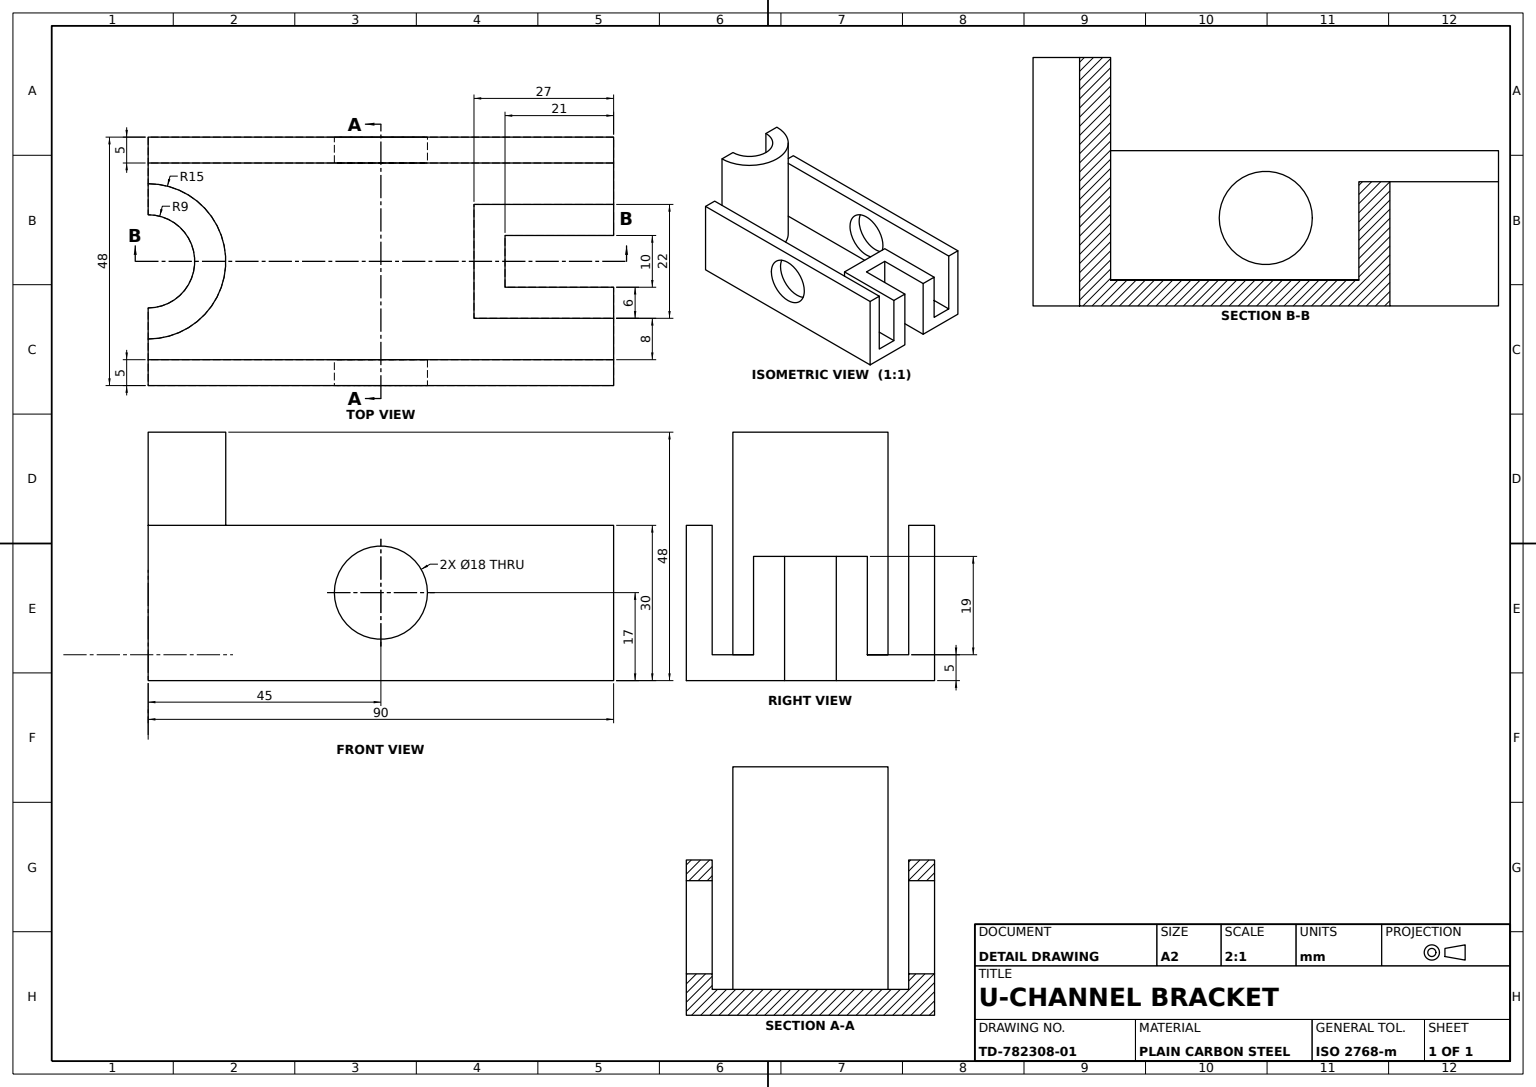
from build123d import *

# Parameters (mm, degrees)
BASE_BLOCK_SKETCH_W         = 90
BASE_BLOCK_SKETCH_H         = 48
BASE_BLOCK_90X48X30_DEPTH   = 30
CHANNEL_SKETCH_W            = 38
CHANNEL_SKETCH_H            = 25
U_CHANNEL_CUT_DEPTH         = 98.857038582
HALF_CYLINDER_POST_30_DEPTH = 48
POST_BORE_SKETCH_R          = 9
POST_BORE_18_DEPTH          = 48
END_TAB_SKETCH_W            = 27
END_TAB_SKETCH_H            = 22
END_TAB_DEPTH               = 19
END_TAB_SLOT_SKETCH_W       = 21
END_TAB_SLOT_SKETCH_H       = 10
END_TAB_SLOT_DEPTH          = 57.364882684
SIDE_HOLE_SKETCH_R          = 9
SIDE_HOLE_18_DEPTH          = 19
OPPOSITE_START              = -19
OPPOSITE_SIDE_HOLE_SKETCH_R = 9
OPPOSITE_SIDE_HOLE_18_DEPTH = 19


with BuildPart() as part:
    # Base Block Sketch → Base Block 90x48x30 (new body)
    with BuildSketch(Plane(origin=(0, 0, 0), x_dir=(1, 0, 0), z_dir=(0, 1, 0))):
        Rectangle(BASE_BLOCK_SKETCH_W, BASE_BLOCK_SKETCH_H)
    extrude(amount=BASE_BLOCK_90X48X30_DEPTH)

    # Channel Sketch → U-Channel Cut (cut, through all)
    with BuildSketch(Plane.ZY.offset(45)):
        with Locations((0, 17.5)):
            Rectangle(CHANNEL_SKETCH_W, CHANNEL_SKETCH_H)
    extrude(amount=-U_CHANNEL_CUT_DEPTH, mode=Mode.SUBTRACT)

    # Half Cylinder Post Sketch → Half Cylinder Post Ø30 (add)
    with BuildSketch(Plane.XZ):
        with BuildLine():
            Line((-45, 15), (-45, -15))
            ThreePointArc((-45, -15), (-30, 0), (-45, 15))
        make_face()
    extrude(amount=-HALF_CYLINDER_POST_30_DEPTH)

    # Post Bore Sketch → Post Bore Ø18 (cut)
    with BuildSketch(Plane(origin=(0, 48, 0), x_dir=(1, 0, 0), z_dir=(0, 1, 0))):
        with Locations((-45, 0)):
            Circle(POST_BORE_SKETCH_R)
    extrude(amount=-POST_BORE_18_DEPTH, mode=Mode.SUBTRACT)

    # End Tab Sketch → End Tab (add)
    with BuildSketch(Plane(origin=(0, 5, 0), x_dir=(1, 0, 0), z_dir=(0, 1, 0))):
        with Locations((31.5, 0)):
            Rectangle(END_TAB_SKETCH_W, END_TAB_SKETCH_H)
    extrude(amount=END_TAB_DEPTH)

    # End Tab Slot Sketch → End Tab Slot (cut, through all)
    with BuildSketch(Plane(origin=(0, 24, 0), x_dir=(1, 0, 0), z_dir=(0, 1, 0))):
        with Locations((34.5, 0)):
            Rectangle(END_TAB_SLOT_SKETCH_W, END_TAB_SLOT_SKETCH_H)
    extrude(amount=-END_TAB_SLOT_DEPTH, mode=Mode.SUBTRACT)

    # Side Hole Sketch → Side Hole Ø18 (cut)
    with BuildSketch(Plane.XY.offset(24)):
        with Locations((0, 17)):
            Circle(SIDE_HOLE_SKETCH_R)
    extrude(amount=-SIDE_HOLE_18_DEPTH, mode=Mode.SUBTRACT)

    # Opposite Side Hole Sketch → Opposite Side Hole Ø18 (cut)
    with BuildSketch(Plane(origin=(0, 0, -24), x_dir=(-1, 0, 0), z_dir=(0, 0, -1)).offset(OPPOSITE_START)):
        with Locations(Location((0, 17, 0), (0, 0, 180))):
            Circle(OPPOSITE_SIDE_HOLE_SKETCH_R)
    extrude(amount=OPPOSITE_SIDE_HOLE_18_DEPTH, mode=Mode.SUBTRACT)


solid = part.part
